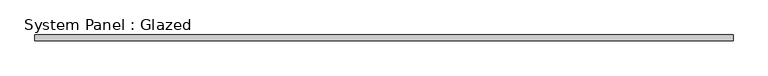
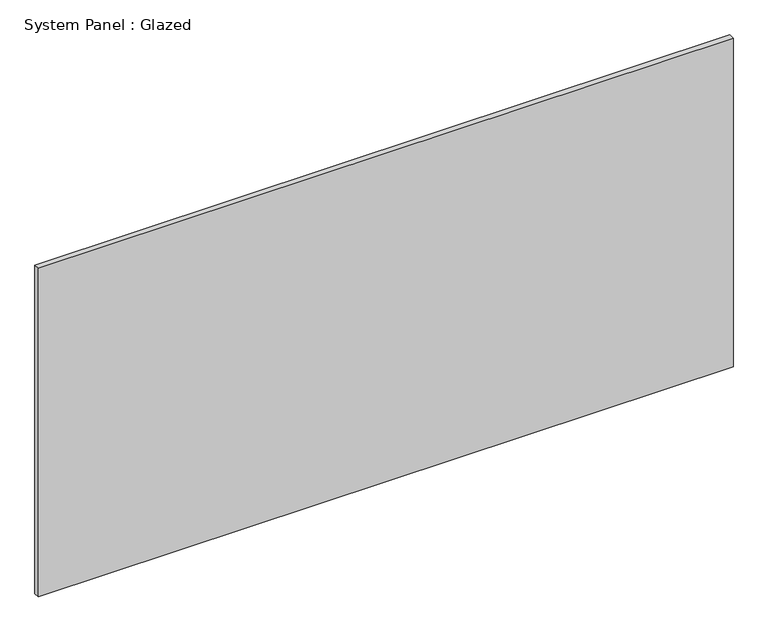
"""IFC4 building model written with IfcOpenShell, lengths in millimetres: plate geometry, System Panel : Glazed."""

from ifc_helpers import new_model, si_unit, origin, origin_with_axes, place, context, project, spatial, polyline, outline, extrude, source, transform, mapped, element, save


def system_panel_glazed_1e57f9bb(model_context):
    return source(origin(), model_context, "Body", "SweptSolid", [
        extrude(outline(polyline([(1524.0000002, 19.05), (-1524.0000002, 19.05), (-1524.0000002, 44.45), (1524.0000002, 44.45), (1524.0000002, 19.05)])), origin_with_axes(), (0.0, 0.0, 1.0), 1524.0),
    ])


if __name__ == "__main__":
    model = new_model("IFC4")
    model_context = context("Model", 3, world=origin())
    ifc_project = project(units=[si_unit("LENGTHUNIT", "METRE", prefix="MILLI")], contexts=[model_context])
    site = spatial("IfcSite", under=ifc_project)
    building = spatial("IfcBuilding", under=site)
    placement = place(None, origin())
    system_panel_glazed_shape = system_panel_glazed_1e57f9bb(model_context)
    element("IfcPlate", 1, ObjectType="System Panel : Glazed", at=placement, inside=building, context=model_context, shape_type="MappedRepresentation", body=[
        mapped(system_panel_glazed_shape, transform((0.0, 0.0, 0.0), x_axis=(1.0, 0.0, 0.0), y_axis=(0.0, 1.0, 0.0), z_axis=(0.0, 0.0, 1.0))),
    ])
    save(model, "model.ifc")

# Revit data of these elements
# Type "System Panel : Glazed"
#   Construction Type Id = "GSP4R"
#   Analytic Construction = "1/8 in Pilkington single glazing"
#   Visual Light Transmittance = 0.9
#   Solar Heat Gain Coefficient = 0.86
#   Heat Transfer Coefficient (U) = 1.18115 BTU/(h·ft²·°F)
#   Define Thermal Properties by = 1
# Element 1 (IfcPlate, "System Panel : Glazed")
#   Materials on its faces: "Glass"
# Materials
#   "Glass": class "Glass", colour RGB 0 128 192, transparency 0.75, Description = "Soda Lime Glass", Cost = 0
